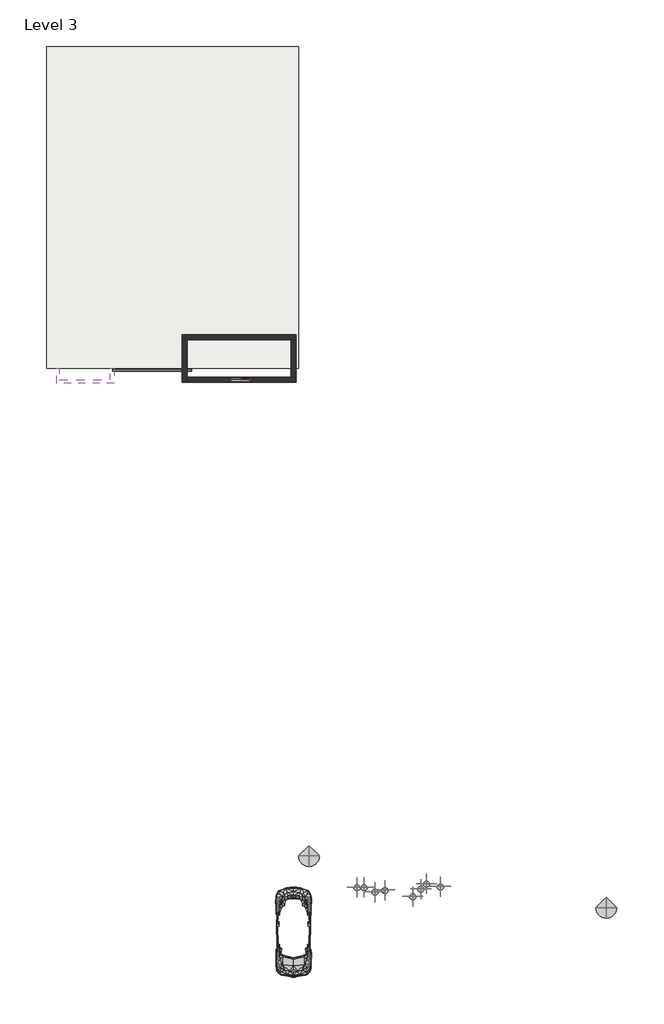
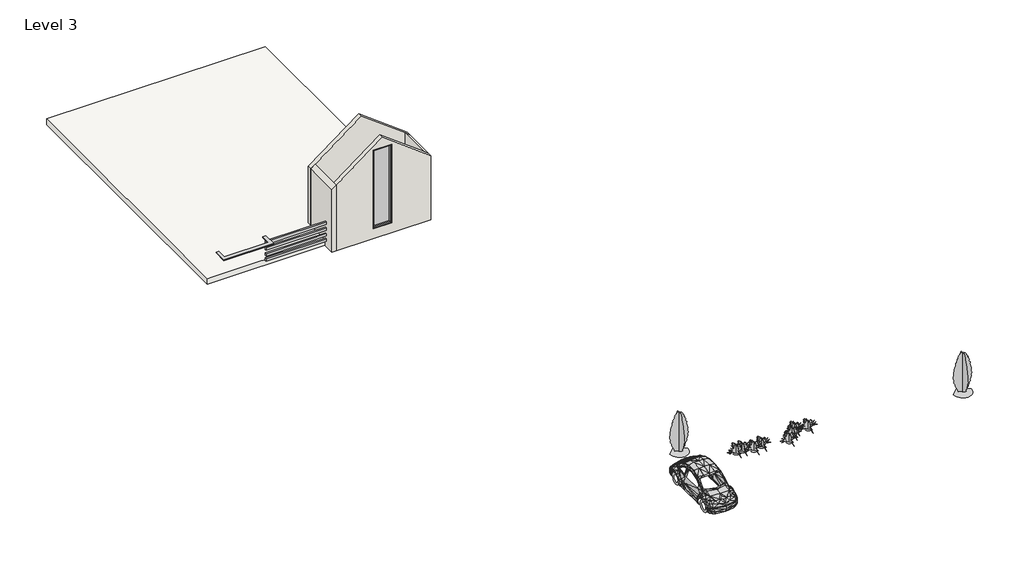
# One storey: 10 geographic elements, 4 members, 4 walls, 3 proxies, 1 plate, 1 roof.
"""IFC4 building model written with IfcOpenShell, lengths in millimetres."""

from ifc_helpers import new_model, si_unit, frame, origin, place, context, project, spatial, polyline, outline, extrude, faceted_brep, transform, mapped, element, save
from components import generic_models_3_generic_models_3_88f68afe, generic_models_4_generic_models_4_79451922, rpc_beetle_rpc_beetle_31f8b51e, rpc_plant_tropical_agave_1_5_93a2a214, rpc_tree_conifer_chinese_juniper_7_1b9786cd, member_e9605c56, member_6420ba3e, system_panel_glazed_14c0cd2a

model = new_model("IFC4")

# Units and contexts
model_context = context("Model", 3, world=origin())
ifc_project = project(units=[si_unit("LENGTHUNIT", "METRE", prefix="MILLI")], contexts=[model_context])

# Site, building, storey
site = spatial("IfcSite", under=ifc_project)
building = spatial("IfcBuilding", under=site)
storey = spatial("IfcBuildingStorey", under=building, Name="Level 3", Elevation=6096.0)

# Proxies
placement = place(None, origin())
generic_models_3_generic_models_3_shape = generic_models_3_generic_models_3_88f68afe(model_context)
element("IfcBuildingElementProxy", 1, Name="Generic Models 3 : Generic Models 3", ObjectType="Generic Models 3 : Generic Models 3", at=placement, inside=storey, context=model_context, shape_type="MappedRepresentation", body=[
    mapped(generic_models_3_generic_models_3_shape, transform((0.0, 0.0, 0.0), x_axis=(1.0, 0.0, 0.0), y_axis=(0.0, 1.0, 0.0), z_axis=(0.0, 0.0, 1.0))),
])
generic_models_4_generic_models_4_shape = generic_models_4_generic_models_4_79451922(model_context)
element("IfcBuildingElementProxy", 2, Name="Generic Models 4 : Generic Models 4", ObjectType="Generic Models 4 : Generic Models 4", at=placement, inside=storey, context=model_context, shape_type="MappedRepresentation", body=[
    mapped(generic_models_4_generic_models_4_shape, transform((0.0, 0.0, 0.0), x_axis=(1.0, 0.0, 0.0), y_axis=(0.0, 1.0, 0.0), z_axis=(0.0, 0.0, 1.0))),
])
rpc_beetle_rpc_beetle_shape = rpc_beetle_rpc_beetle_31f8b51e(model_context)
element("IfcBuildingElementProxy", 3, Name="RPC Beetle : RPC Beetle", ObjectType="RPC Beetle : RPC Beetle", at=placement, inside=storey, context=model_context, shape_type="MappedRepresentation", body=[
    mapped(rpc_beetle_rpc_beetle_shape, transform((-5833.7281629, -38483.6678064, 6096.0), x_axis=(-1.0, 0.0, 0.0), y_axis=(0.0, -1.0, 0.0), z_axis=(0.0, 0.0, 1.0))),
])

# Geographic elements
rpc_plant_tropical_agave_1_5_shape = rpc_plant_tropical_agave_1_5_93a2a214(model_context)
element("IfcGeographicElement", 4, ObjectType="RPC Plant - Tropical : Agave - 1.5'", at=placement, inside=storey, context=model_context, shape_type="MappedRepresentation", body=[
    mapped(rpc_plant_tropical_agave_1_5_shape, transform((-3027.0281629, -37721.6678064, 6096.0), x_axis=(1.0, 0.0, 0.0), y_axis=(0.0, 1.0, 0.0), z_axis=(0.0, 0.0, 1.0))),
])
element("IfcGeographicElement", 5, ObjectType="RPC Plant - Tropical : Agave - 1.5'", at=placement, inside=storey, context=model_context, shape_type="MappedRepresentation", body=[
    mapped(rpc_plant_tropical_agave_1_5_shape, transform((-2722.2281629, -37721.6678064, 6096.0), x_axis=(1.0, 0.0, 0.0), y_axis=(0.0, 1.0, 0.0), z_axis=(0.0, 0.0, 1.0))),
])
element("IfcGeographicElement", 6, ObjectType="RPC Plant - Tropical : Agave - 1.5'", at=placement, inside=storey, context=model_context, shape_type="MappedRepresentation", body=[
    mapped(rpc_plant_tropical_agave_1_5_shape, transform((-2239.6281629, -37924.8678064, 6096.0), x_axis=(1.0, 0.0, 0.0), y_axis=(0.0, 1.0, 0.0), z_axis=(0.0, 0.0, 1.0))),
])
element("IfcGeographicElement", 7, ObjectType="RPC Plant - Tropical : Agave - 1.5'", at=placement, inside=storey, context=model_context, shape_type="MappedRepresentation", body=[
    mapped(rpc_plant_tropical_agave_1_5_shape, transform((-1807.8281629, -37848.6678064, 6096.0), x_axis=(1.0, 0.0, 0.0), y_axis=(0.0, 1.0, 0.0), z_axis=(0.0, 0.0, 1.0))),
])
element("IfcGeographicElement", 8, ObjectType="RPC Plant - Tropical : Agave - 1.5'", at=placement, inside=storey, context=model_context, shape_type="MappedRepresentation", body=[
    mapped(rpc_plant_tropical_agave_1_5_shape, transform((-575.9281629, -38128.0678064, 6096.0), x_axis=(1.0, 0.0, 0.0), y_axis=(0.0, 1.0, 0.0), z_axis=(0.0, 0.0, 1.0))),
])
element("IfcGeographicElement", 9, ObjectType="RPC Plant - Tropical : Agave - 1.5'", at=placement, inside=storey, context=model_context, shape_type="MappedRepresentation", body=[
    mapped(rpc_plant_tropical_agave_1_5_shape, transform((-220.3281629, -37797.8678064, 6096.0), x_axis=(1.0, 0.0, 0.0), y_axis=(0.0, 1.0, 0.0), z_axis=(0.0, 0.0, 1.0))),
])
element("IfcGeographicElement", 10, ObjectType="RPC Plant - Tropical : Agave - 1.5'", at=placement, inside=storey, context=model_context, shape_type="MappedRepresentation", body=[
    mapped(rpc_plant_tropical_agave_1_5_shape, transform((33.6718371, -37569.2678064, 6096.0), x_axis=(1.0, 0.0, 0.0), y_axis=(0.0, 1.0, 0.0), z_axis=(0.0, 0.0, 1.0))),
])
element("IfcGeographicElement", 11, ObjectType="RPC Plant - Tropical : Agave - 1.5'", at=placement, inside=storey, context=model_context, shape_type="MappedRepresentation", body=[
    mapped(rpc_plant_tropical_agave_1_5_shape, transform((643.2718371, -37696.2678064, 6096.0), x_axis=(1.0, 0.0, 0.0), y_axis=(0.0, 1.0, 0.0), z_axis=(0.0, 0.0, 1.0))),
])
rpc_tree_conifer_chinese_juniper_7_shape = rpc_tree_conifer_chinese_juniper_7_1b9786cd(model_context)
element("IfcGeographicElement", 12, ObjectType="RPC Tree - Conifer : Chinese Juniper - 7'", at=placement, inside=storey, context=model_context, shape_type="MappedRepresentation", body=[
    mapped(rpc_tree_conifer_chinese_juniper_7_shape, transform((-5148.124834, -36350.0678064, 6096.0), x_axis=(1.0, 0.0, 0.0), y_axis=(0.0, 1.0, 0.0), z_axis=(0.0, 0.0, 1.0))),
])
element("IfcGeographicElement", 13, ObjectType="RPC Tree - Conifer : Chinese Juniper - 7'", at=placement, inside=storey, context=model_context, shape_type="MappedRepresentation", body=[
    mapped(rpc_tree_conifer_chinese_juniper_7_shape, transform((7958.275166, -38636.0678064, 6096.0), x_axis=(1.0, 0.0, 0.0), y_axis=(0.0, 1.0, 0.0), z_axis=(0.0, 0.0, 1.0))),
])

# Members
member_shape = member_e9605c56(model_context)
element("IfcMember", 14, ObjectType="Rectangular Mullion : 2.5\" x 5\" rectangular", at=placement, inside=storey, context=model_context, shape_type="MappedRepresentation", body=[
    mapped(member_shape, transform((-7764.1281629, -15356.9678064, 10857.0372822), x_axis=(0.0, 0.0, 1.0), y_axis=(0.0, -1.0, 0.0), z_axis=(1.0, 0.0, 0.0))),
])
element("IfcMember", 15, ObjectType="Rectangular Mullion : 2.5\" x 5\" rectangular", at=placement, inside=storey, context=model_context, shape_type="MappedRepresentation", body=[
    mapped(member_shape, transform((-8589.6281629, -15356.9678064, 6626.9948921), x_axis=(0.0, 0.0, -1.0), y_axis=(0.0, -1.0, 0.0), z_axis=(-1.0, 0.0, 0.0))),
])
member_2_shape = member_6420ba3e(model_context)
element("IfcMember", 16, ObjectType="Rectangular Mullion : 2.5\" x 5\" rectangular", at=placement, inside=storey, context=model_context, shape_type="MappedRepresentation", body=[
    mapped(member_2_shape, transform((-8653.1281629, -15356.9678064, 10857.0372822), x_axis=(-1.0, 0.0, 0.0), y_axis=(0.0, -1.0, 0.0), z_axis=(0.0, 0.0, 1.0))),
])
element("IfcMember", 17, ObjectType="Rectangular Mullion : 2.5\" x 5\" rectangular", at=placement, inside=storey, context=model_context, shape_type="MappedRepresentation", body=[
    mapped(member_2_shape, transform((-7700.6281629, -15356.9678064, 6626.9948921), x_axis=(1.0, 0.0, 0.0), y_axis=(0.0, -1.0, 0.0), z_axis=(0.0, 0.0, -1.0))),
])

# Plate
system_panel_glazed_shape = system_panel_glazed_14c0cd2a(model_context)
element("IfcPlate", 18, ObjectType="System Panel : Glazed", at=placement, inside=storey, context=model_context, shape_type="MappedRepresentation", body=[
    mapped(system_panel_glazed_shape, transform((-8176.8781629, -15356.9678064, 6690.4948921), x_axis=(1.0, 0.0, 0.0), y_axis=(0.0, 1.0, 0.0), z_axis=(0.0, 0.0, 1.0))),
])

# Roof
element("IfcRoof", 19, ObjectType="Generic - 12\"", at=placement, inside=storey, context=model_context, shape_type="SweptSolid", body=[
    extrude(outline(polyline([(-16730.3281629, -675.7678064), (-5605.1281629, -675.7678064), (-5605.1281629, -14848.9678064), (-16730.3281629, -14848.9678064), (-16730.3281629, -675.7678064)])), frame((0.0, 0.0, 6096.0), z_axis=(0.0, 0.0, 1.0), x_axis=(1.0, 0.0, 0.0)), (0.0, 0.0, 1.0), 304.8),
])

# Walls
element("IfcWall", 20, ObjectType="9\"", at=placement, inside=storey, context=model_context, shape_type="Brep", body=[
    faceted_brep([(-10748.6281629, -13604.3678064, 6096.0), (-10520.0281629, -13604.3678064, 6096.0), (-5948.0281629, -13604.3678064, 6096.0), (-5719.4281629, -13604.3678064, 6096.0), (-5719.4281629, -13604.3678064, 9539.3581213), (-5948.0281629, -13604.3678064, 9710.8081213), (-8184.0352072, -13604.3678064, 11387.8134045), (-10520.0281629, -13604.3678064, 9635.8186877), (-10748.6281629, -13604.3678064, 9464.3686877), (-10748.6281629, -13375.7678064, 6096.0), (-10748.6281629, -13375.7678064, 9464.3686877), (-8184.0352072, -13375.7678064, 11387.8134045), (-5719.4281629, -13375.7678064, 9539.3581213), (-5719.4281629, -13375.7678064, 6096.0)], [[[0, 1, 2, 3, 4, 5, 6, 7, 8]], [[9, 10, 11, 12, 13]], [[3, 2, 1, 0, 9, 13]], [[0, 8, 10, 9]], [[4, 3, 13, 12]], [[8, 7, 6, 11, 10]], [[6, 5, 4, 12, 11]]]),
])
element("IfcWall", 21, ObjectType="9\"", at=placement, inside=storey, context=model_context, shape_type="Brep", body=[
    faceted_brep([(-10748.6281629, -13604.3678064, 6096.0), (-10748.6281629, -15471.2678064, 6096.0), (-10748.6281629, -15471.2678064, 9464.3686877), (-10748.6281629, -13604.3678064, 9464.3686877), (-10520.0281629, -13604.3678064, 6096.0), (-10520.0281629, -13604.3678064, 9635.8186877), (-10520.0281629, -15242.6678064, 9635.8186877), (-10520.0281629, -15471.2678064, 9635.8186877), (-10520.0281629, -15471.2678064, 6096.0), (-10520.0281629, -15242.6678064, 6096.0)], [[[0, 1, 2, 3]], [[4, 5, 6, 7, 8, 9]], [[1, 0, 4, 9, 8]], [[0, 3, 5, 4]], [[2, 1, 8, 7]], [[3, 2, 7, 6, 5]]]),
])
element("IfcWall", 22, ObjectType="9\"", at=placement, inside=storey, context=model_context, shape_type="Brep", body=[
    faceted_brep([(-10520.0281629, -15471.2678064, 6096.0), (-5719.4281629, -15471.2678064, 6096.0), (-5719.4281629, -15471.2678064, 9539.3581213), (-8184.0352072, -15471.2678064, 11387.8134045), (-10520.0281629, -15471.2678064, 9635.8186877), (-8653.1281629, -15471.2678064, 6626.9948921), (-8653.1281629, -15471.2678064, 10857.0372822), (-7700.6281629, -15471.2678064, 10857.0372822), (-7700.6281629, -15471.2678064, 6626.9948921), (-5719.4281629, -15242.6678064, 6096.0), (-5948.0281629, -15242.6678064, 6096.0), (-10520.0281629, -15242.6678064, 6096.0), (-10520.0281629, -15242.6678064, 9635.8186877), (-8184.0352072, -15242.6678064, 11387.8134045), (-5948.0281629, -15242.6678064, 9710.8081213), (-5719.4281629, -15242.6678064, 9539.3581213), (-8653.1281629, -15242.6678064, 10857.0372822), (-8653.1281629, -15242.6678064, 6626.9948921), (-7700.6281629, -15242.6678064, 6626.9948921), (-7700.6281629, -15242.6678064, 10857.0372822)], [[[0, 1, 2, 3, 4], [5, 6, 7, 8]], [[9, 10, 11, 12, 13, 14, 15], [16, 17, 18, 19]], [[1, 0, 11, 10, 9]], [[0, 4, 12, 11]], [[2, 1, 9, 15]], [[12, 4, 3, 13]], [[2, 15, 14, 13, 3]], [[5, 17, 16, 6]], [[6, 16, 19, 7]], [[7, 19, 18, 8]], [[17, 5, 8, 18]]]),
])
element("IfcWall", 23, ObjectType="9\"", at=placement, inside=storey, context=model_context, shape_type="SweptSolid", body=[
    extrude(outline(polyline([(6096.0, -5719.4281629), (9539.3581213, -5719.4281629), (9710.8081213, -5948.0281629), (6096.0, -5948.0281629), (6096.0, -5719.4281629)])), frame((0.0, -15242.6678064, 0.0), z_axis=(0.0, 1.0, 0.0), x_axis=(0.0, 0.0, 1.0)), (0.0, 0.0, 1.0), 1638.3),
])

save(model, "model.ifc")

# Revit data of these elements
# Type "RPC Beetle : RPC Beetle"
#   built-in parameter 1005198 = "{2, 15},{39, RPC-16-0U6E-L4EG-ENH1-J3KF-SVEL-0TX4-C0},{1, 0},{1, 0},{2, 36},{1, 8},{5, Color},{1, 0},{1, 0},{3, 0.8},{3, 0.8},{3, 0.8},{1, 8},{7, BBoxMin},{1, 0},{1, 0},{1, 0},{1, 0},{1, 0},{1, 8},{7, BBoxMax},{1, 0},{1, 0},{1, 0},{1, 0},{1, 0},{2, 11},{9, RPCTypeId},{1, 0},{1, 0},{39, RPC-16-0U6E-L4EG-ENH1-J3KF-SVEL-0TX4-C0},{1, 6},{14, RPCPlantHeight},{1, 0},{1, 0},{7, 4.91667},{2, 11},{20, AdvancedUIDefinition},{1, 0},{1, 0},{0, },{2, 11},{10, AssetLibID},{1, 0},{1, 0},{36, 4D3F6E72-3F99-4203-98E9-AF80B3C7A7A4},{2, 11},{10, BaseSchema},{1, 0},{1, 0},{9, RPCSchema},{2, 11},{12, ExchangeGUID},{1, 0},{1, 0},{0, },{1, 2},{6, Hidden},{1, 0},{1, 0},{1, 0},{2, 11},{12, LocalizedUID},{1, 0},{1, 0},{0, },{1, 4},{11, RPCCategory},{1, 0},{1, 0},{1, 0},{2, 11},{8, RPCImage},{1, 0},{1, 0},{0, },{1, 4},{13, SchemaVersion},{1, 0},{1, 0},{1, 4},{2, 11},{12, UIDefinition},{1, 0},{1, 0},{0, },{2, 11},{6, UIName},{1, 0},{1, 0},{39, RPC-16-0U6E-L4EG-ENH1-J3KF-SVEL-0TX4-C0},{2, 11},{11, VersionGUID},{1, 0},{1, 0},{9, RPCSchema},{2, 11},{9, assettype},{1, 0},{1, 0},{11, RPCGeometry},{2, 11},{11, description},{1, 0},{1, 0},{0, },{2, 11},{9, localname},{1, 0},{1, 0},{3, RPC},{2, 11},{9, localtype},{1, 0},{1, 0},{3, RPC},{1, 4},{8, revision},{1, 0},{1, 0},{1, 1},{2, 11},{9, thumbnail},{1, 0},{1, 0},{0, },{1, 4},{7, version},{1, 0},{1, 0},{1, 1},{2, 14},{6, Height},{1, 0},{1, 0},{7, 4.91667},{1, 2},{20, RPC_Cast Reflections},{1, 0},{1, 0},{1, 1},{1, 4},{16, RPC_Transparency},{1, 0},{1, 0},{2, 18},{1, 4},{11, RPC_Tinting},{1, 0},{1, 0},{2, 50},{1, 2},{15, RPC_Use Tinting},{1, 0},{1, 0},{1, 0},{1, 2},{17, RPC_License Plate},{1, 0},{1, 0},{1, 0},{2, 11},{25, RPC_License Plate Texture},{1, 0},{1, 0},{64, __RPC:/object data/textures/car/plate/textures/default/rgb/0/0/0},{2, 11},{27, RPC_i_License Plate Texture},{1, 0},{1, 0},{0, },{1, 2},{16, RPC_Custom Plate},{1, 0},{1, 0},{1, 0},{2, 11},{27, RPC_License Plate File Name},{1, 0},{1, 0},{0, },{2, 11},{7, keyword},{1, 0},{1, 0},{27, :Geometry:RPC:VW Beetle [4]},{2, 11},{8, category},{1, 0},{1, 0},{21, :Auto_Economy/Midsize},{21, assetlibrary_base.fbx},{1, 5},"
#   built-in parameter 1005195 = "RPC-16-0U6E-L4EG-ENH1-J3KF-SVEL-0TX4-C0"
#   Height = 0
# Type "RPC Plant - Tropical : Agave - 1.5'"
#   built-in parameter 1005198 = "{2, 15},{39, RPC-16-G1GJ-63FX-7K5P-N000-ST1L-LVER-AU},{1, 0},{1, 0},{2, 35},{1, 8},{5, Color},{1, 0},{1, 0},{3, 0.8},{3, 0.8},{3, 0.8},{1, 8},{7, BBoxMin},{1, 0},{1, 0},{1, 0},{1, 0},{1, 0},{1, 8},{7, BBoxMax},{1, 0},{1, 0},{1, 0},{1, 0},{1, 0},{2, 11},{9, RPCTypeId},{1, 0},{1, 0},{39, RPC-16-G1GJ-63FX-7K5P-N000-ST1L-LVER-AU},{1, 6},{14, RPCPlantHeight},{1, 0},{1, 0},{3, 1.5},{2, 11},{7, keyword},{1, 0},{1, 0},{88, :Geometry:RPC:Agave:agave:agave americana marginata:mesqual:south western:tropical:plant},{2, 11},{8, category},{1, 0},{1, 0},{17, :Plants [General]},{2, 11},{12, LocalizedUID},{1, 0},{1, 0},{5, Agave},{2, 14},{6, Height},{1, 0},{1, 0},{3, 1.5},{1, 2},{16, Cast Reflections},{1, 0},{1, 0},{1, 0},{1, 2},{12, Cast Shadows},{1, 0},{1, 0},{1, 1},{1, 2},{9, Lock View},{1, 0},{1, 0},{1, 0},{1, 4},{5, ViewC},{1, 0},{1, 0},{1, 0},{2, 11},{20, AdvancedUIDefinition},{1, 0},{1, 0},{0, },{2, 11},{10, AssetLibID},{1, 0},{1, 0},{36, 4D3F6E72-3F99-4203-98E9-AF80B3C7A7A4},{2, 11},{10, BaseSchema},{1, 0},{1, 0},{9, RPCSchema},{2, 11},{12, ExchangeGUID},{1, 0},{1, 0},{0, },{1, 2},{6, Hidden},{1, 0},{1, 0},{1, 0},{1, 4},{11, RPCCategory},{1, 0},{1, 0},{1, 0},{2, 11},{8, RPCImage},{1, 0},{1, 0},{0, },{1, 4},{13, SchemaVersion},{1, 0},{1, 0},{1, 4},{2, 11},{12, UIDefinition},{1, 0},{1, 0},{0, },{2, 11},{6, UIName},{1, 0},{1, 0},{39, RPC-16-G1GJ-63FX-7K5P-N000-ST1L-LVER-AU},{2, 11},{11, VersionGUID},{1, 0},{1, 0},{9, RPCSchema},{2, 11},{9, assettype},{1, 0},{1, 0},{11, RPCGeometry},{2, 11},{11, description},{1, 0},{1, 0},{0, },{2, 11},{9, localname},{1, 0},{1, 0},{3, RPC},{2, 11},{9, localtype},{1, 0},{1, 0},{3, RPC},{1, 4},{8, revision},{1, 0},{1, 0},{1, 1},{2, 11},{9, thumbnail},{1, 0},{1, 0},{0, },{1, 4},{7, version},{1, 0},{1, 0},{1, 1},{1, 2},{20, RPC_Cast Reflections},{1, 0},{1, 0},{1, 1},{1, 2},{16, RPC_Cast Shadows},{1, 0},{1, 0},{1, 1},{1, 2},{13, RPC_Lock View},{1, 0},{1, 0},{1, 0},{1, 4},{9, RPC_ViewC},{1, 0},{1, 0},{1, 0},{21, assetlibrary_base.fbx},{1, 5},"
#   built-in parameter 1005195 = "RPC-16-G1GJ-63FX-7K5P-N000-ST1L-LVER-AU"
#   Type Comments = "Agave"
#   Assembly Code = "G2050500"
#   Height = 1' - 6"
#   Default Elevation = 0
# Type "RPC Tree - Conifer : Chinese Juniper - 7'"
#   built-in parameter 1005198 = "{2, 15},{39, RPC-16-FUM3-UUQ0-UBF0-N000-ST1L-LVER-AU},{1, 0},{1, 0},{2, 35},{1, 8},{5, Color},{1, 0},{1, 0},{3, 0.8},{3, 0.8},{3, 0.8},{1, 8},{7, BBoxMin},{1, 0},{1, 0},{1, 0},{1, 0},{1, 0},{1, 8},{7, BBoxMax},{1, 0},{1, 0},{1, 0},{1, 0},{1, 0},{2, 11},{9, RPCTypeId},{1, 0},{1, 0},{39, RPC-16-FUM3-UUQ0-UBF0-N000-ST1L-LVER-AU},{1, 6},{14, RPCPlantHeight},{1, 0},{1, 0},{1, 7},{2, 11},{7, keyword},{1, 0},{1, 0},{96, :Geometry:RPC:Chinese Juniper:juniperus chinensis:chinese:juniper:cupressaceae:conifer:evergreen},{2, 11},{8, category},{1, 0},{1, 0},{16, :Trees [General]},{2, 11},{12, LocalizedUID},{1, 0},{1, 0},{15, Chinese Juniper},{2, 14},{6, Height},{1, 0},{1, 0},{1, 7},{1, 2},{16, Cast Reflections},{1, 0},{1, 0},{1, 0},{1, 2},{12, Cast Shadows},{1, 0},{1, 0},{1, 1},{1, 2},{9, Lock View},{1, 0},{1, 0},{1, 0},{1, 4},{5, ViewC},{1, 0},{1, 0},{1, 0},{2, 11},{20, AdvancedUIDefinition},{1, 0},{1, 0},{0, },{2, 11},{10, AssetLibID},{1, 0},{1, 0},{36, 4D3F6E72-3F99-4203-98E9-AF80B3C7A7A4},{2, 11},{10, BaseSchema},{1, 0},{1, 0},{9, RPCSchema},{2, 11},{12, ExchangeGUID},{1, 0},{1, 0},{0, },{1, 2},{6, Hidden},{1, 0},{1, 0},{1, 0},{1, 4},{11, RPCCategory},{1, 0},{1, 0},{1, 0},{2, 11},{8, RPCImage},{1, 0},{1, 0},{0, },{1, 4},{13, SchemaVersion},{1, 0},{1, 0},{1, 4},{2, 11},{12, UIDefinition},{1, 0},{1, 0},{0, },{2, 11},{6, UIName},{1, 0},{1, 0},{39, RPC-16-FUM3-UUQ0-UBF0-N000-ST1L-LVER-AU},{2, 11},{11, VersionGUID},{1, 0},{1, 0},{9, RPCSchema},{2, 11},{9, assettype},{1, 0},{1, 0},{11, RPCGeometry},{2, 11},{11, description},{1, 0},{1, 0},{0, },{2, 11},{9, localname},{1, 0},{1, 0},{3, RPC},{2, 11},{9, localtype},{1, 0},{1, 0},{3, RPC},{1, 4},{8, revision},{1, 0},{1, 0},{1, 1},{2, 11},{9, thumbnail},{1, 0},{1, 0},{0, },{1, 4},{7, version},{1, 0},{1, 0},{1, 1},{1, 2},{20, RPC_Cast Reflections},{1, 0},{1, 0},{1, 1},{1, 2},{16, RPC_Cast Shadows},{1, 0},{1, 0},{1, 1},{1, 2},{13, RPC_Lock View},{1, 0},{1, 0},{1, 0},{1, 4},{9, RPC_ViewC},{1, 0},{1, 0},{1, 0},{21, assetlibrary_base.fbx},{1, 5},"
#   built-in parameter 1005195 = "RPC-16-FUM3-UUQ0-UBF0-N000-ST1L-LVER-AU"
#   Type Comments = "Chinese Juniper"
#   Assembly Code = "G2050500"
#   Height = 7' - 0"
#   Description = (empty or 0)
#   Default Elevation = 0
# Type "Rectangular Mullion : 2.5\" x 5\" rectangular"
#   built-in parameter 1007304 = 0.416667 (stored number, unit not read)
#   built-in parameter 1007301 = 0.104167 (stored number, unit not read)
#   built-in parameter 1007300 = 0.104167 (stored number, unit not read)
# Type "System Panel : Glazed"
#   Construction Type Id = "GSP4R"
#   Analytic Construction = "1/8 in Pilkington single glazing"
#   Visual Light Transmittance = 0.9
#   Solar Heat Gain Coefficient = 0.86
#   Heat Transfer Coefficient (U) = 1.18115 BTU/(h·ft²·°F)
#   Define Thermal Properties by = 1
# Type "Generic - 12\""
#   Assembly Code = "B1020"
#   Layers, outside or top first: 1' - 0" no material (function 1)
# Type "9\""
#   Assembly Code = "B2010"
#   Layers, outside or top first: 0' - 9" no material (function 1)
# Element 1 (IfcBuildingElementProxy, "Generic Models 3 : Generic Models 3")
#   Phase Created = New Construction
# Element 2 (IfcBuildingElementProxy, "Generic Models 4 : Generic Models 4")
#   Phase Created = New Construction
# Element 3 (IfcBuildingElementProxy, "RPC Beetle : RPC Beetle")
#   Phase Created = New Construction
# Elements 4, 5, 6, 7, 8, 9, 10, 11 (IfcGeographicElement, "RPC Plant - Tropical : Agave - 1.5'")
#   Phase Created = New Construction
# Elements 12, 13 (IfcGeographicElement, "RPC Tree - Conifer : Chinese Juniper - 7'")
#   Phase Created = New Construction
# Elements 14, 15, 16, 17 (IfcMember, "Rectangular Mullion : 2.5\" x 5\" rectangular")
#   Phase Created = New Construction
#   Materials on its faces: "Aluminum"
# Element 18 (IfcPlate, "System Panel : Glazed")
#   Phase Created = New Construction
#   Materials on its faces: "Glass"
# Element 19 (IfcRoof, "Generic - 12\"")
#   built-in parameter 1001705 = 21 (stored number, unit not read)
#   built-in parameter 1001710 = 33615
#   Phase Created = New Construction
#   Materials on its faces: "Default Roof"
# Elements 20, 21, 22, 23 (IfcWall, "9\"")
#   Top Offset = 0' - 0"
#   Base Offset = 0' - 0"
#   Unconnected Height = 10' - 0"
#   wall height = 10' - 0"
#   Phase Created = New Construction
#   Base Constraint = Level 3
#   Materials on its faces: "Default Wall"
# Materials
#   "Aluminum": class "Metal", colour RGB 247 247 247, transparency 0, Description = "Aluminum 6061", Cost = 0
#   "Glass": class "Glass", colour RGB 0 128 192, transparency 0.75, Description = "Soda Lime Glass", Cost = 0
#   "Default Roof": colour RGB 88 101 114, transparency 0, Cost = 0
#   "Default Wall": colour RGB 128 128 128, transparency 0, Cost = 0
